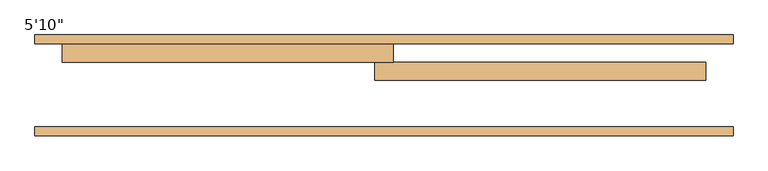
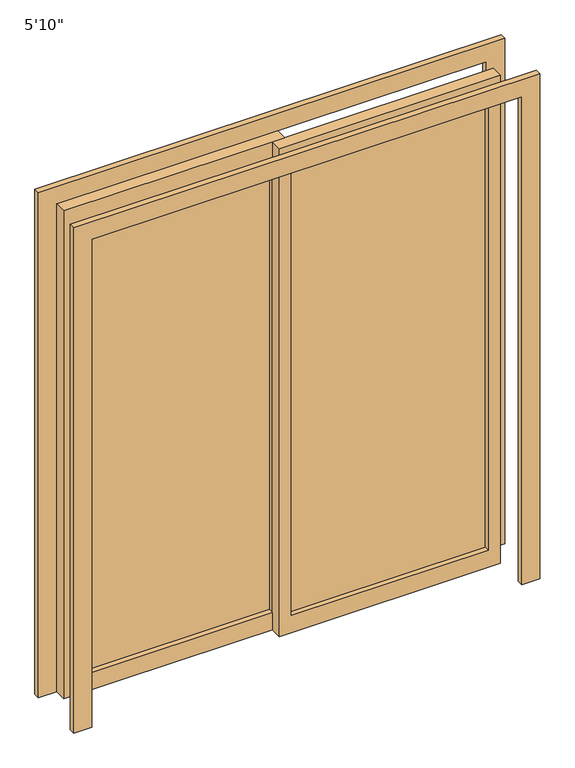
"""IFC4 building model written with IfcOpenShell, lengths in millimetres: door geometry."""

from ifc_helpers import new_model, si_unit, frame, origin, place, context, project, spatial, polyline, outline, extrude, source, transform, mapped, element, save


def door_510b0506(model_context):
    return source(origin(), model_context, "Body", "SweptSolid", [
        extrude(outline(polyline([(0.0, 964.0), (2209.0, 964.0), (2209.0, -964.0), (0.0, -964.0), (0.0, -889.0), (2134.0, -889.0), (2134.0, 889.0), (0.0, 889.0), (0.0, 964.0)])), frame((0.0, 241.3, 0.0), z_axis=(0.0, 1.0, 0.0), x_axis=(0.0, 0.0, 1.0)), (0.0, 0.0, 1.0), 25.0),
        extrude(outline(polyline([(0.0, -964.0), (0.0, -889.0), (2134.0, -889.0), (2134.0, 889.0), (0.0, 889.0), (0.0, 964.0), (2209.0, 964.0), (2209.0, -964.0), (0.0, -964.0)])), frame((0.0, -12.3, 0.0), z_axis=(0.0, 1.0, 0.0), x_axis=(0.0, 0.0, 1.0)), (0.0, 0.0, 1.0), 25.0),
        extrude(outline(polyline([(2134.0, 25.4), (2134.0, -889.0), (0.0, -889.0), (0.0, 25.4), (2134.0, 25.4)]), holes=[polyline([(2059.0, -24.6), (75.0, -24.6), (75.0, -839.0), (2059.0, -839.0), (2059.0, -24.6)])]), frame((0.0, 191.3, 0.0), z_axis=(0.0, 1.0, 0.0), x_axis=(0.0, 0.0, 1.0)), (0.0, 0.0, 1.0), 50.0),
        extrude(outline(polyline([(-839.0, 219.475), (-24.6, 219.475), (-24.6, 213.125), (-839.0, 213.125), (-839.0, 219.475)])), frame((0.0, 0.0, 75.0), z_axis=(0.0, 0.0, 1.0), x_axis=(1.0, 0.0, 0.0)), (0.0, 0.0, 1.0), 1984.0),
        extrude(outline(polyline([(2134.0, -25.4), (0.0, -25.4), (0.0, 889.0), (2134.0, 889.0), (2134.0, -25.4)]), holes=[polyline([(2059.0, 24.6), (2059.0, 839.0), (75.0, 839.0), (75.0, 24.6), (2059.0, 24.6)])]), frame((0.0, 141.3, 0.0), z_axis=(0.0, 1.0, 0.0), x_axis=(0.0, 0.0, 1.0)), (0.0, 0.0, 1.0), 50.0),
        extrude(outline(polyline([(25.4, 169.475), (839.0, 169.475), (839.0, 163.125), (25.4, 163.125), (25.4, 169.475)])), frame((0.0, 0.0, 75.0), z_axis=(0.0, 0.0, 1.0), x_axis=(1.0, 0.0, 0.0)), (0.0, 0.0, 1.0), 1984.0),
    ])


if __name__ == "__main__":
    model = new_model("IFC4")
    model_context = context("Model", 3, world=origin())
    ifc_project = project(units=[si_unit("LENGTHUNIT", "METRE", prefix="MILLI")], contexts=[model_context])
    site = spatial("IfcSite", under=ifc_project)
    building = spatial("IfcBuilding", under=site)
    placement = place(None, origin())
    door_shape = door_510b0506(model_context)
    element("IfcDoor", 1, ObjectType="5'10\"", at=placement, inside=building, context=model_context, shape_type="MappedRepresentation", body=[
        mapped(door_shape, transform((0.0, 0.0, 0.0), x_axis=(1.0, 0.0, 0.0), y_axis=(0.0, 1.0, 0.0), z_axis=(0.0, 0.0, 1.0))),
    ])
    save(model, "model.ifc")

# Revit data of these elements
# Type "5'10\""
#   Type Mark = "55"
#   Thickness = 0' - 1.9685"
#   Height = 7' - 0.01575"
#   Anchura de barandal = 0' - 2.95276"
#   Anchura de montante = 0' - 1.9685"
#   Proyección cubrejuntas ext. = 0' - 0.98425"
#   Proyección cubrejuntas int. = 0' - 0.98425"
#   Anchura de cubrejuntas = 0' - 2.95276"
#   Width = 5' - 10"
#   Material de puerta = Puerta - Panel
#   Function = (empty or 0)
#   Assembly Code = ""
#   Wall Closure = (empty or 0)
# Element 1 (IfcDoor, "5'10\"")
#   Materials on its faces: "Puerta - Panel", "Cristal"
# Materials
#   "Puerta - Panel": class "Madera", colour RGB 210 159 95, transparency 0
#   "Cristal": class "Vidrio", colour RGB 0 0 255, transparency 0.75
